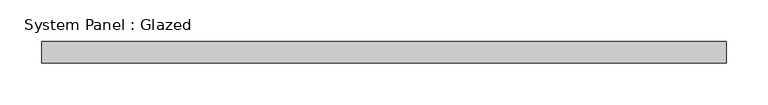
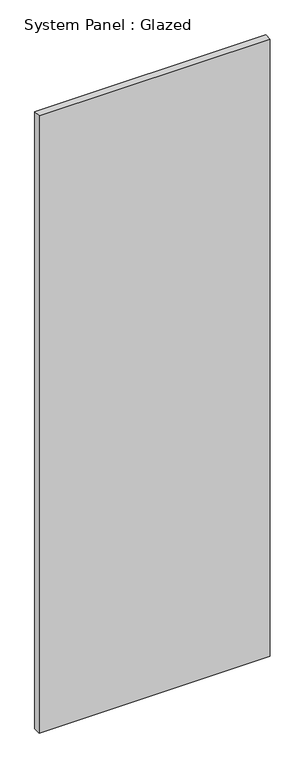
"""IFC4 building model written with IfcOpenShell, lengths in millimetres: plate geometry, System Panel : Glazed."""

from ifc_helpers import new_model, si_unit, origin, origin_with_axes, place, context, project, spatial, polyline, outline, extrude, source, transform, mapped, element, save


def system_panel_glazed_061c0ed8(model_context):
    return source(origin(), model_context, "Body", "SweptSolid", [
        extrude(outline(polyline([(409.575, 19.05), (-409.575, 19.05), (-409.575, 44.45), (409.575, 44.45), (409.575, 19.05)])), origin_with_axes(), (0.0, 0.0, 1.0), 2311.4),
    ])


if __name__ == "__main__":
    model = new_model("IFC4")
    model_context = context("Model", 3, world=origin())
    ifc_project = project(units=[si_unit("LENGTHUNIT", "METRE", prefix="MILLI")], contexts=[model_context])
    site = spatial("IfcSite", under=ifc_project)
    building = spatial("IfcBuilding", under=site)
    placement = place(None, origin())
    system_panel_glazed_shape = system_panel_glazed_061c0ed8(model_context)
    element("IfcPlate", 1, ObjectType="System Panel : Glazed", at=placement, inside=building, context=model_context, shape_type="MappedRepresentation", body=[
        mapped(system_panel_glazed_shape, transform((0.0, 0.0, 0.0), x_axis=(1.0, 0.0, 0.0), y_axis=(0.0, 1.0, 0.0), z_axis=(0.0, 0.0, 1.0))),
    ])
    save(model, "model.ifc")

# Revit data of these elements
# Type "System Panel : Glazed"
#   Construction Type Id = "GSP4R"
#   Analytic Construction = "1/8 in Pilkington single glazing"
#   Visual Light Transmittance = 0.9
#   Solar Heat Gain Coefficient = 0.86
#   Heat Transfer Coefficient (U) = 1.18115 BTU/(h·ft²·°F)
#   Define Thermal Properties by = 1
# Element 1 (IfcPlate, "System Panel : Glazed")
#   Materials on its faces: "Glass"
# Materials
#   "Glass": class "Glass", colour RGB 0 128 192, transparency 0.75, Description = "Soda Lime Glass", Cost = 0
